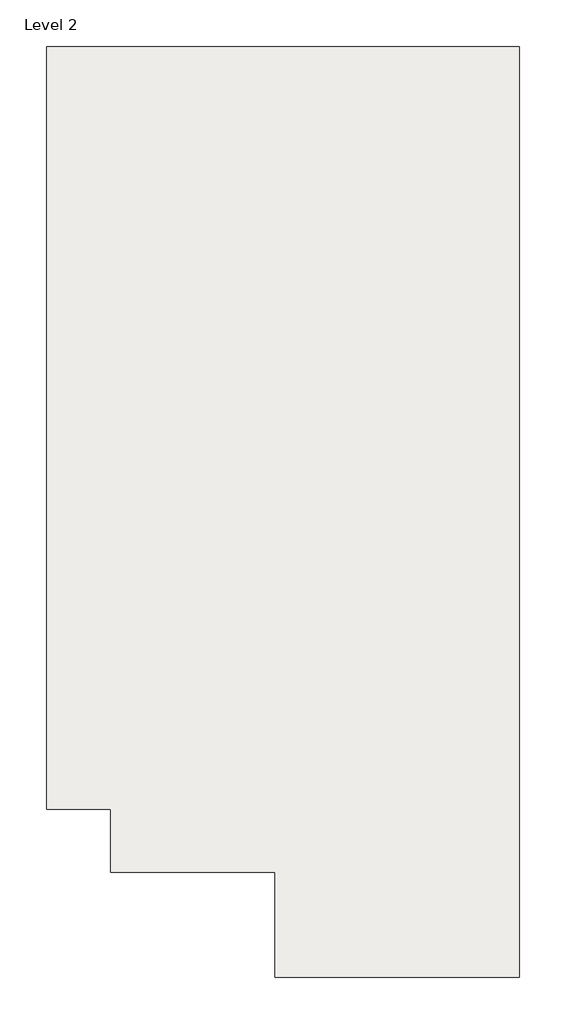
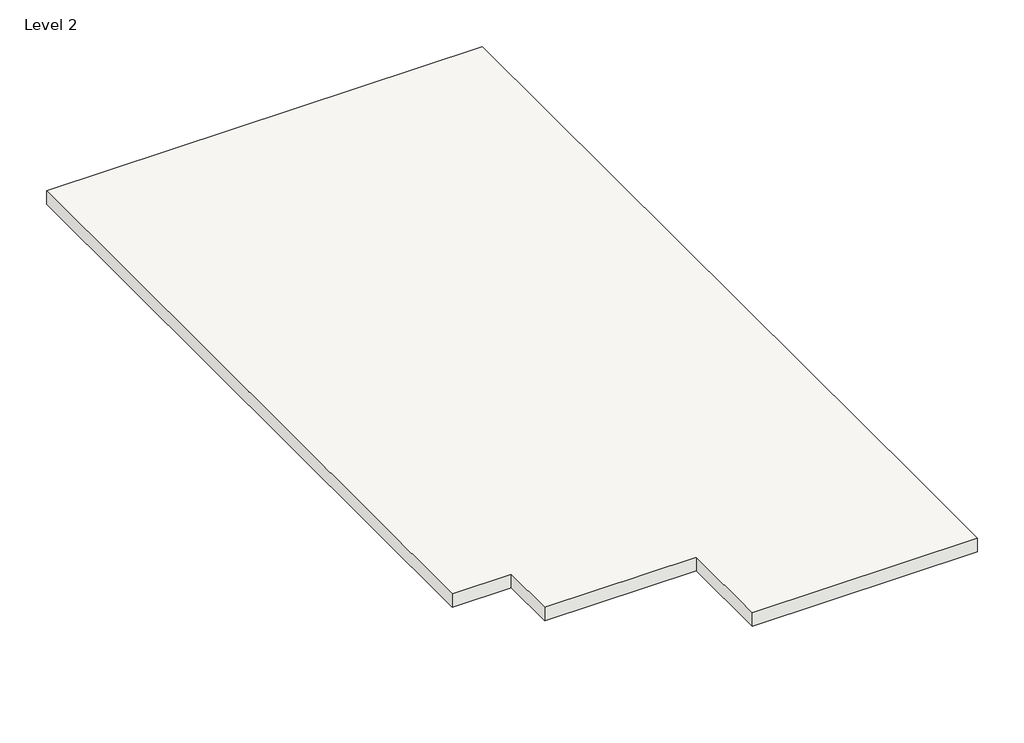
# One storey: 1 roof.
"""IFC4 building model written with IfcOpenShell, lengths in millimetres."""

from ifc_helpers import new_model, si_unit, frame, origin, place, context, project, spatial, polyline, outline, extrude, element, save

model = new_model("IFC4")

# Units and contexts
model_context = context("Model", 3, world=origin())
ifc_project = project(units=[si_unit("LENGTHUNIT", "METRE", prefix="MILLI")], contexts=[model_context])

# Site, building, storey
site = spatial("IfcSite", under=ifc_project)
building = spatial("IfcBuilding", under=site)
storey = spatial("IfcBuildingStorey", under=building, Name="Level 2", Elevation=3048.0)

# Roof
placement = place(None, origin())
element("IfcRoof", 1, ObjectType="Generic - 12\"", at=placement, inside=storey, context=model_context, shape_type="SweptSolid", body=[
    extrude(outline(polyline([(-14681.0021832, 12967.4104001), (-5333.8021832, 12967.4104001), (-5333.8021832, 953.2104001), (-5333.8021832, -3161.5895999), (-5333.8021832, -5422.1895999), (-10159.8021832, -5422.1895999), (-10159.8021832, -3339.3895999), (-13411.0021832, -3339.3895999), (-13411.0021832, -2094.7895999), (-14681.0021832, -2094.7895999), (-14681.0021832, 12967.4104001)])), frame((0.0, 0.0, 3048.0), z_axis=(0.0, 0.0, 1.0), x_axis=(1.0, 0.0, 0.0)), (0.0, 0.0, 1.0), 304.8),
])

save(model, "model.ifc")

# Revit data of these elements
# Type "Generic - 12\""
#   Assembly Code = "B1020"
#   Layers, outside or top first: 1' - 0" "Brick, Soldier Course" (function 1)
# Element 1 (IfcRoof, "Generic - 12\"")
#   built-in parameter 1001705 = 11 (stored number, unit not read)
#   built-in parameter 1001710 = 33615
#   Phase Created = New Construction
#   Materials on its faces: "Brick, Soldier Course"
# Materials
#   "Brick, Soldier Course": class "Masonry", colour RGB 170 98 104, transparency 0, Description = "Common brick soldier coursed", Cost = 0
